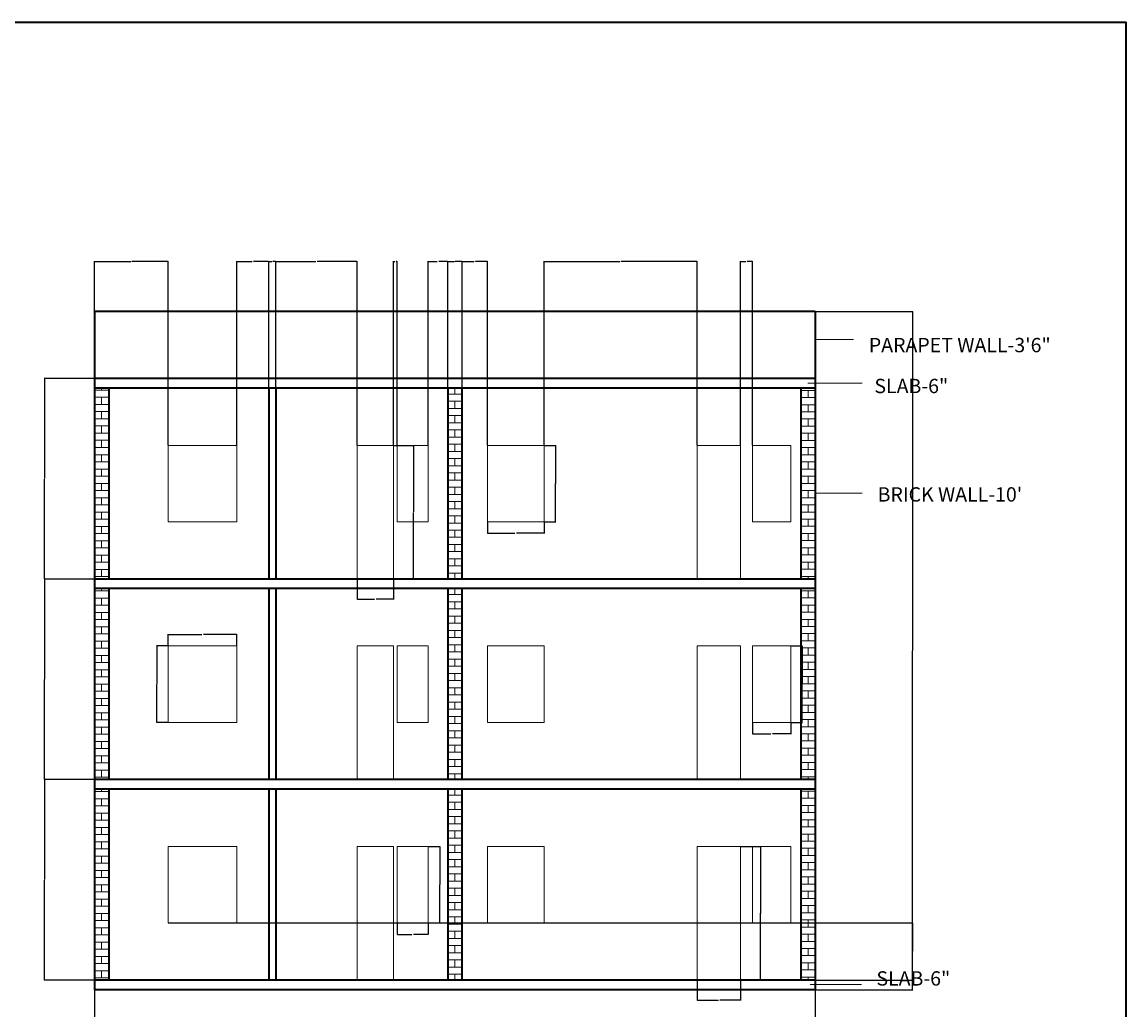
# Model space of a CAD drawing. Units: inches. Extents: x 2250 to 3629, y 982 to 2740.
# Tile 12 of 12: x 2936 to 3629, y 2119 to 2740. Entities that reach past the tile are written whole.
import ezdxf

# ---------------------------------------------------------------- set-up
doc = ezdxf.new("R2010")
doc.units = ezdxf.units.IN
for name, color, linetype, lineweight in [('A-ANNO-DIMS', 2, 'Continuous', 18), ('A-ANNO-TEXT', 7, 'Continuous', 18), ('A-ANNO-TTLB', 7, 'Continuous', 35), ('A-SECT', 7, 'Continuous', 35), ('A-SECT-DOOR', 3, 'Continuous', 18), ('A-SECT-GLAZ', 4, 'Continuous', 18), ('A-WALL-PATT', 252, 'Continuous', 13)]:
    doc.layers.add(name, color=color, linetype=linetype, lineweight=lineweight)
doc.styles.get("Standard").update_dxf_attribs({"font": 'arial.ttf'})
doc.dimstyles.get("Standard").update_dxf_attribs({"dimtxt": 0.18, "dimasz": 0.18, "dimexe": 0.18, "dimexo": 0.0625, "dimgap": 0.09, "dimtad": 0, "dimtih": 1, "dimtoh": 1, "dimdec": 4, "dimzin": 0, "dimdsep": 46, "dimtxsty": 'Standard', "dimcen": 0.09, "dimadec": 0, "dimazin": 0, "dimtfac": 1, "dimtdec": 4, "dimtofl": 0, "dimtmove": 0, "dimatfit": 3, "dimfxl": 1, "dimtolj": 1, "dimtzin": 0, "dimarcsym": 0})

# ---------------------------------------------------------------- blocks, each defined once
blk = doc.blocks.new('SEC-WIN-24x48')
for p, q in [((0, 48), (0, 0)), ((24, 48), (0, 48)), ((24, 48), (24, 0)), ((24, 0), (0, 0))]:
    blk.add_line(p, q)
blk = doc.blocks.new('SEC-WIN-35p52x48')
for p, q in [((0, 48), (0, 0)), ((35.52, 48), (0, 48)), ((35.52, 48), (35.52, 0)), ((35.52, 0), (0, 0))]:
    blk.add_line(p, q)
blk = doc.blocks.new('SEC-WIN-19p52x48')
for p, q in [((0, 48), (0, 0)), ((19.52, 48), (0, 48)), ((19.52, 48), (19.52, 0)), ((19.52, 0), (0, 0))]:
    blk.add_line(p, q)
blk = doc.blocks.new('SEC-WIN-43p24x48')
for p, q in [((0, 48), (0, 0)), ((43.24, 48), (0, 48)), ((43.24, 48), (43.24, 0)), ((43.24, 0), (0, 0))]:
    blk.add_line(p, q)
blk = doc.blocks.new('SEC-DOOR-27p25x84')
for p, q in [((0, 84), (0, 0)), ((27.25, 84), (0, 84)), ((27.25, 84), (27.25, 0))]:
    blk.add_line(p, q)
blk = doc.blocks.new('SEC-DOOR-22p88x84')
for p, q in [((0, 84), (0, 0)), ((22.88, 84), (0, 84)), ((22.88, 84), (22.88, 0))]:
    blk.add_line(p, q)
blk = doc.blocks.new('*D157')
at = {"layer": 'A-ANNO-DIMS', "color": 0, "lineweight": -2, "transparency": 16777216}
for p, q in [((3418.84, 2347.7), (3426.15, 2347.7)), ((3425.97, 2347.52), (3425.97, 2323.88)), ((3425.97, 2299.88), (3425.97, 2323.52)), ((3418.84, 2299.7), (3426.15, 2299.7))]:
    blk.add_line(p, q, dxfattribs=at)
at = {"layer": 'A-ANNO-DIMS', "color": 0, "transparency": 16777216}
for points in [[(3425.94, 2347.52), (3426, 2347.52), (3425.97, 2347.7)], [(3425.94, 2299.88), (3426, 2299.88), (3425.97, 2299.7)]]:
    blk.add_solid(points, dxfattribs=at)
at = {"layer": 'Defpoints', "color": 0, "transparency": 16777216}
for p in [(3418.77, 2347.7), (3425.97, 2347.7), (3418.77, 2299.7)]:
    blk.add_point(p, dxfattribs=at)
at = {"layer": 'A-ANNO-DIMS', "color": 0, "transparency": 16777216, "insert": (3425.97, 2323.7), "char_height": 0.18, "attachment_point": 5}
blk.add_mtext('\\A1;WINDOW 48 TYP.', dxfattribs=at)
blk = doc.blocks.new('*D158')
at = {"layer": 'A-ANNO-DIMS', "color": 0, "lineweight": -2, "transparency": 16777216}
for p, q in [((3394.77, 2299.64), (3394.77, 2292.32)), ((3418.77, 2299.64), (3418.77, 2292.32)), ((3394.95, 2292.5), (3406.24, 2292.5)), ((3418.59, 2292.5), (3407.3, 2292.5))]:
    blk.add_line(p, q, dxfattribs=at)
at = {"layer": 'A-ANNO-DIMS', "color": 0, "transparency": 16777216}
for points in [[(3394.95, 2292.53), (3394.95, 2292.47), (3394.77, 2292.5)], [(3418.59, 2292.53), (3418.59, 2292.47), (3418.77, 2292.5)]]:
    blk.add_solid(points, dxfattribs=at)
at = {"layer": 'Defpoints', "color": 0, "transparency": 16777216}
for p in [(3394.77, 2299.7), (3418.77, 2299.7), (3418.77, 2292.5)]:
    blk.add_point(p, dxfattribs=at)
at = {"layer": 'A-ANNO-DIMS', "color": 0, "transparency": 16777216, "insert": (3406.77, 2292.5), "char_height": 0.18, "attachment_point": 5}
blk.add_mtext('\\A1;24 TYP.', dxfattribs=at)
blk = doc.blocks.new('*D159')
at = {"layer": 'A-ANNO-DIMS', "color": 0, "lineweight": -2, "transparency": 16777216}
for p, q in [((3263.8, 2473.7), (3271.12, 2473.7)), ((3270.94, 2473.52), (3270.94, 2449.88)), ((3270.94, 2425.88), (3270.94, 2449.52)), ((3263.8, 2425.7), (3271.12, 2425.7))]:
    blk.add_line(p, q, dxfattribs=at)
at = {"layer": 'A-ANNO-DIMS', "color": 0, "transparency": 16777216}
for points in [[(3270.91, 2473.52), (3270.97, 2473.52), (3270.94, 2473.7)], [(3270.91, 2425.88), (3270.97, 2425.88), (3270.94, 2425.7)]]:
    blk.add_solid(points, dxfattribs=at)
at = {"layer": 'Defpoints', "color": 0, "transparency": 16777216}
for p in [(3263.74, 2473.7), (3270.94, 2473.7), (3263.74, 2425.7)]:
    blk.add_point(p, dxfattribs=at)
at = {"layer": 'A-ANNO-DIMS', "color": 0, "transparency": 16777216, "insert": (3270.94, 2449.7), "char_height": 0.18, "attachment_point": 5}
blk.add_mtext('\\A1;WINDOW 48 TYP.', dxfattribs=at)
blk = doc.blocks.new('*D160')
at = {"layer": 'A-ANNO-DIMS', "color": 0, "lineweight": -2, "transparency": 16777216}
for p, q in [((3228.22, 2425.64), (3228.22, 2418.32)), ((3263.74, 2425.64), (3263.74, 2418.32)), ((3228.4, 2418.5), (3245.45, 2418.5)), ((3263.56, 2418.5), (3246.51, 2418.5))]:
    blk.add_line(p, q, dxfattribs=at)
at = {"layer": 'A-ANNO-DIMS', "color": 0, "transparency": 16777216}
for points in [[(3228.4, 2418.53), (3228.4, 2418.47), (3228.22, 2418.5)], [(3263.56, 2418.53), (3263.56, 2418.47), (3263.74, 2418.5)]]:
    blk.add_solid(points, dxfattribs=at)
at = {"layer": 'Defpoints', "color": 0, "transparency": 16777216}
for p in [(3228.22, 2425.7), (3263.74, 2425.7), (3263.74, 2418.5)]:
    blk.add_point(p, dxfattribs=at)
at = {"layer": 'A-ANNO-DIMS', "color": 0, "transparency": 16777216, "insert": (3245.98, 2418.5), "char_height": 0.18, "attachment_point": 5}
blk.add_mtext('\\A1;36 TYP.', dxfattribs=at)
blk = doc.blocks.new('*D161')
at = {"layer": 'A-ANNO-DIMS', "color": 0, "lineweight": -2, "transparency": 16777216}
for p, q in [((3191.07, 2221.7), (3198.39, 2221.7)), ((3198.21, 2221.52), (3198.21, 2197.88)), ((3198.21, 2173.88), (3198.21, 2197.52)), ((3191.07, 2173.7), (3198.39, 2173.7))]:
    blk.add_line(p, q, dxfattribs=at)
at = {"layer": 'A-ANNO-DIMS', "color": 0, "transparency": 16777216}
for points in [[(3198.18, 2221.52), (3198.24, 2221.52), (3198.21, 2221.7)], [(3198.18, 2173.88), (3198.24, 2173.88), (3198.21, 2173.7)]]:
    blk.add_solid(points, dxfattribs=at)
at = {"layer": 'Defpoints', "color": 0, "transparency": 16777216}
for p in [(3191.01, 2221.7), (3198.21, 2221.7), (3191.01, 2173.7)]:
    blk.add_point(p, dxfattribs=at)
at = {"layer": 'A-ANNO-DIMS', "color": 0, "transparency": 16777216, "insert": (3198.21, 2197.7), "char_height": 0.18, "attachment_point": 5}
blk.add_mtext('\\A1;WINDOW 48 TYP.', dxfattribs=at)
blk = doc.blocks.new('*D162')
at = {"layer": 'A-ANNO-DIMS', "color": 0, "lineweight": -2, "transparency": 16777216}
for p, q in [((3171.49, 2173.64), (3171.49, 2166.32)), ((3191.01, 2173.64), (3191.01, 2166.32)), ((3171.67, 2166.5), (3180.72, 2166.5)), ((3190.83, 2166.5), (3181.78, 2166.5))]:
    blk.add_line(p, q, dxfattribs=at)
at = {"layer": 'A-ANNO-DIMS', "color": 0, "transparency": 16777216}
for points in [[(3171.67, 2166.53), (3171.67, 2166.47), (3171.49, 2166.5)], [(3190.83, 2166.53), (3190.83, 2166.47), (3191.01, 2166.5)]]:
    blk.add_solid(points, dxfattribs=at)
at = {"layer": 'Defpoints', "color": 0, "transparency": 16777216}
for p in [(3171.49, 2173.7), (3191.01, 2173.7), (3191.01, 2166.5)]:
    blk.add_point(p, dxfattribs=at)
at = {"layer": 'A-ANNO-DIMS', "color": 0, "transparency": 16777216, "insert": (3181.25, 2166.5), "char_height": 0.18, "attachment_point": 5}
blk.add_mtext('\\A1;20 TYP.', dxfattribs=at)
blk = doc.blocks.new('*D163')
at = {"layer": 'A-ANNO-DIMS', "color": 0, "lineweight": -2, "transparency": 16777216}
for p, q in [((3027.45, 2347.7), (3020.13, 2347.7)), ((3020.31, 2347.52), (3020.31, 2323.88)), ((3020.31, 2299.88), (3020.31, 2323.52)), ((3027.45, 2299.7), (3020.13, 2299.7))]:
    blk.add_line(p, q, dxfattribs=at)
at = {"layer": 'A-ANNO-DIMS', "color": 0, "transparency": 16777216}
for points in [[(3020.28, 2347.52), (3020.34, 2347.52), (3020.31, 2347.7)], [(3020.28, 2299.88), (3020.34, 2299.88), (3020.31, 2299.7)]]:
    blk.add_solid(points, dxfattribs=at)
at = {"layer": 'Defpoints', "color": 0, "transparency": 16777216}
for p in [(3027.51, 2347.7), (3020.31, 2299.7), (3027.51, 2299.7)]:
    blk.add_point(p, dxfattribs=at)
at = {"layer": 'A-ANNO-DIMS', "color": 0, "transparency": 16777216, "insert": (3020.31, 2323.7), "char_height": 0.18, "attachment_point": 5}
blk.add_mtext('\\A1;WINDOW 48 TYP.', dxfattribs=at)
blk = doc.blocks.new('*D164')
at = {"layer": 'A-ANNO-DIMS', "color": 0, "lineweight": -2, "transparency": 16777216}
for p, q in [((3027.51, 2347.76), (3027.51, 2355.08)), ((3027.69, 2354.9), (3048.6, 2354.9)), ((3070.58, 2354.9), (3049.67, 2354.9)), ((3070.76, 2347.76), (3070.76, 2355.08))]:
    blk.add_line(p, q, dxfattribs=at)
at = {"layer": 'A-ANNO-DIMS', "color": 0, "transparency": 16777216}
for points in [[(3027.69, 2354.93), (3027.69, 2354.87), (3027.51, 2354.9)], [(3070.58, 2354.93), (3070.58, 2354.87), (3070.76, 2354.9)]]:
    blk.add_solid(points, dxfattribs=at)
at = {"layer": 'Defpoints', "color": 0, "transparency": 16777216}
for p in [(3027.51, 2354.9), (3027.51, 2347.7), (3070.76, 2347.7)]:
    blk.add_point(p, dxfattribs=at)
at = {"layer": 'A-ANNO-DIMS', "color": 0, "transparency": 16777216, "insert": (3049.14, 2354.9), "char_height": 0.18, "attachment_point": 5}
blk.add_mtext('\\A1;43 TYP.', dxfattribs=at)
blk = doc.blocks.new('*D165')
at = {"layer": 'A-ANNO-DIMS', "color": 0, "lineweight": -2, "transparency": 16777216}
for p, q in [((3387.34, 2221.7), (3400.06, 2221.7)), ((3399.88, 2221.52), (3399.88, 2179.88)), ((3399.88, 2137.88), (3399.88, 2179.52)), ((3387.34, 2137.7), (3400.06, 2137.7))]:
    blk.add_line(p, q, dxfattribs=at)
at = {"layer": 'A-ANNO-DIMS', "color": 0, "transparency": 16777216}
for points in [[(3399.85, 2221.52), (3399.91, 2221.52), (3399.88, 2221.7)], [(3399.85, 2137.88), (3399.91, 2137.88), (3399.88, 2137.7)]]:
    blk.add_solid(points, dxfattribs=at)
at = {"layer": 'Defpoints', "color": 0, "transparency": 16777216}
for p in [(3387.28, 2221.7), (3399.88, 2221.7), (3387.28, 2137.7)]:
    blk.add_point(p, dxfattribs=at)
at = {"layer": 'A-ANNO-DIMS', "color": 0, "transparency": 16777216, "insert": (3399.88, 2179.7), "char_height": 0.18, "attachment_point": 5}
blk.add_mtext('\\A1;DOOR 84 TYP.', dxfattribs=at)
blk = doc.blocks.new('*D166')
at = {"layer": 'A-ANNO-DIMS', "color": 0, "lineweight": -2, "transparency": 16777216}
for p, q in [((3360.02, 2137.64), (3360.02, 2124.92)), ((3387.28, 2137.64), (3387.28, 2124.92)), ((3360.2, 2125.1), (3373.12, 2125.1)), ((3387.1, 2125.1), (3374.18, 2125.1))]:
    blk.add_line(p, q, dxfattribs=at)
at = {"layer": 'A-ANNO-DIMS', "color": 0, "transparency": 16777216}
for points in [[(3360.2, 2125.13), (3360.2, 2125.07), (3360.02, 2125.1)], [(3387.1, 2125.13), (3387.1, 2125.07), (3387.28, 2125.1)]]:
    blk.add_solid(points, dxfattribs=at)
at = {"layer": 'Defpoints', "color": 0, "transparency": 16777216}
for p in [(3360.02, 2137.7), (3387.28, 2137.7), (3387.28, 2125.1)]:
    blk.add_point(p, dxfattribs=at)
at = {"layer": 'A-ANNO-DIMS', "color": 0, "transparency": 16777216, "insert": (3373.65, 2125.1), "char_height": 0.18, "attachment_point": 5}
blk.add_mtext('\\A1;27 TYP.', dxfattribs=at)
blk = doc.blocks.new('*D167')
at = {"layer": 'A-ANNO-DIMS', "color": 0, "lineweight": -2, "transparency": 16777216}
for p, q in [((3169.27, 2473.7), (3181.99, 2473.7)), ((3181.81, 2473.52), (3181.81, 2431.88)), ((3181.81, 2389.88), (3181.81, 2431.52)), ((3169.27, 2389.7), (3181.99, 2389.7))]:
    blk.add_line(p, q, dxfattribs=at)
at = {"layer": 'A-ANNO-DIMS', "color": 0, "transparency": 16777216}
for points in [[(3181.78, 2473.52), (3181.84, 2473.52), (3181.81, 2473.7)], [(3181.78, 2389.88), (3181.84, 2389.88), (3181.81, 2389.7)]]:
    blk.add_solid(points, dxfattribs=at)
at = {"layer": 'Defpoints', "color": 0, "transparency": 16777216}
for p in [(3169.21, 2473.7), (3181.81, 2473.7), (3169.21, 2389.7)]:
    blk.add_point(p, dxfattribs=at)
at = {"layer": 'A-ANNO-DIMS', "color": 0, "transparency": 16777216, "insert": (3181.81, 2431.7), "char_height": 0.18, "attachment_point": 5}
blk.add_mtext('\\A1;DOOR 84 TYP.', dxfattribs=at)
blk = doc.blocks.new('*D168')
at = {"layer": 'A-ANNO-DIMS', "color": 0, "lineweight": -2, "transparency": 16777216}
for p, q in [((3146.34, 2389.64), (3146.34, 2376.92)), ((3169.21, 2389.64), (3169.21, 2376.92)), ((3146.52, 2377.1), (3157.24, 2377.1)), ((3169.03, 2377.1), (3158.3, 2377.1))]:
    blk.add_line(p, q, dxfattribs=at)
at = {"layer": 'A-ANNO-DIMS', "color": 0, "transparency": 16777216}
for points in [[(3146.52, 2377.13), (3146.52, 2377.07), (3146.34, 2377.1)], [(3169.03, 2377.13), (3169.03, 2377.07), (3169.21, 2377.1)]]:
    blk.add_solid(points, dxfattribs=at)
at = {"layer": 'Defpoints', "color": 0, "transparency": 16777216}
for p in [(3146.34, 2389.7), (3169.21, 2389.7), (3169.21, 2377.1)]:
    blk.add_point(p, dxfattribs=at)
at = {"layer": 'A-ANNO-DIMS', "color": 0, "transparency": 16777216, "insert": (3157.77, 2377.1), "char_height": 0.18, "attachment_point": 5}
blk.add_mtext('\\A1;23 TYP.', dxfattribs=at)
blk = doc.blocks.new('*D188')
at = {"layer": 'A-ANNO-DIMS', "color": 0, "lineweight": -2, "transparency": 16777216}
for p, q in [((2981.23, 2131.64), (2981.23, 2056.9)), ((3434.23, 2131.64), (3434.23, 2056.9)), ((2981.41, 2057.08), (3207.43, 2057.08)), ((3434.05, 2057.08), (3208.02, 2057.08))]:
    blk.add_line(p, q, dxfattribs=at)
at = {"layer": 'A-ANNO-DIMS', "color": 0, "transparency": 16777216}
for points in [[(2981.41, 2057.11), (2981.41, 2057.05), (2981.23, 2057.08)], [(3434.05, 2057.11), (3434.05, 2057.05), (3434.23, 2057.08)]]:
    blk.add_solid(points, dxfattribs=at)
at = {"layer": 'Defpoints', "color": 0, "transparency": 16777216}
for p in [(2981.23, 2131.7), (3434.23, 2131.7), (3434.23, 2057.08)]:
    blk.add_point(p, dxfattribs=at)
at = {"layer": 'A-ANNO-DIMS', "color": 0, "transparency": 16777216, "insert": (3207.73, 2057.08), "char_height": 0.18, "attachment_point": 5}
blk.add_mtext('\\A1;453', dxfattribs=at)
blk = doc.blocks.new('*D189')
at = {"layer": 'A-ANNO-DIMS', "color": 0, "lineweight": -2, "transparency": 16777216}
for p, q in [((3434.29, 2557.7), (3495.46, 2557.7)), ((3495.28, 2557.52), (3495.28, 2344.88)), ((3495.28, 2131.88), (3495.28, 2344.52)), ((3434.29, 2131.7), (3495.46, 2131.7))]:
    blk.add_line(p, q, dxfattribs=at)
at = {"layer": 'A-ANNO-DIMS', "color": 0, "transparency": 16777216}
for points in [[(3495.25, 2557.52), (3495.31, 2557.52), (3495.28, 2557.7)], [(3495.25, 2131.88), (3495.31, 2131.88), (3495.28, 2131.7)]]:
    blk.add_solid(points, dxfattribs=at)
at = {"layer": 'Defpoints', "color": 0, "transparency": 16777216}
for p in [(3434.23, 2557.7), (3495.28, 2557.7), (3434.23, 2131.7)]:
    blk.add_point(p, dxfattribs=at)
at = {"layer": 'A-ANNO-DIMS', "color": 0, "transparency": 16777216, "insert": (3495.28, 2344.7), "char_height": 0.18, "attachment_point": 5}
blk.add_mtext('\\A1;426', dxfattribs=at)
blk = doc.blocks.new('*D190')
at = {"layer": 'A-ANNO-DIMS', "color": 0, "lineweight": -2, "transparency": 16777216}
for p, q in [((2981.16, 2263.7), (2949.55, 2263.7)), ((2949.73, 2263.52), (2949.73, 2200.88)), ((2949.73, 2137.88), (2949.73, 2200.52)), ((2981.16, 2137.7), (2949.55, 2137.7))]:
    blk.add_line(p, q, dxfattribs=at)
at = {"layer": 'A-ANNO-DIMS', "color": 0, "transparency": 16777216}
for points in [[(2949.7, 2263.52), (2949.76, 2263.52), (2949.73, 2263.7)], [(2949.7, 2137.88), (2949.76, 2137.88), (2949.73, 2137.7)]]:
    blk.add_solid(points, dxfattribs=at)
at = {"layer": 'Defpoints', "color": 0, "transparency": 16777216}
for p in [(2949.73, 2263.7), (2981.23, 2263.7), (2981.23, 2137.7)]:
    blk.add_point(p, dxfattribs=at)
at = {"layer": 'A-ANNO-DIMS', "color": 0, "transparency": 16777216, "insert": (2949.73, 2200.7), "char_height": 0.18, "attachment_point": 5}
blk.add_mtext('\\A1;126', dxfattribs=at)
blk = doc.blocks.new('*D191')
at = {"layer": 'A-ANNO-DIMS', "color": 0, "lineweight": -2, "transparency": 16777216}
for p, q in [((2981.16, 2389.7), (2949.55, 2389.7)), ((2949.73, 2389.52), (2949.73, 2326.88)), ((2949.73, 2263.88), (2949.73, 2326.52)), ((2981.16, 2263.7), (2949.55, 2263.7))]:
    blk.add_line(p, q, dxfattribs=at)
at = {"layer": 'A-ANNO-DIMS', "color": 0, "transparency": 16777216}
for points in [[(2949.7, 2389.52), (2949.76, 2389.52), (2949.73, 2389.7)], [(2949.7, 2263.88), (2949.76, 2263.88), (2949.73, 2263.7)]]:
    blk.add_solid(points, dxfattribs=at)
at = {"layer": 'Defpoints', "color": 0, "transparency": 16777216}
for p in [(2949.73, 2389.7), (2981.23, 2389.7), (2981.23, 2263.7)]:
    blk.add_point(p, dxfattribs=at)
at = {"layer": 'A-ANNO-DIMS', "color": 0, "transparency": 16777216, "insert": (2949.73, 2326.7), "char_height": 0.18, "attachment_point": 5}
blk.add_mtext('\\A1;126', dxfattribs=at)
blk = doc.blocks.new('*D192')
at = {"layer": 'A-ANNO-DIMS', "color": 0, "lineweight": -2, "transparency": 16777216}
for p, q in [((2981.16, 2515.7), (2949.55, 2515.7)), ((2949.73, 2515.52), (2949.73, 2452.88)), ((2949.73, 2389.88), (2949.73, 2452.52)), ((2981.16, 2389.7), (2949.55, 2389.7))]:
    blk.add_line(p, q, dxfattribs=at)
at = {"layer": 'A-ANNO-DIMS', "color": 0, "transparency": 16777216}
for points in [[(2949.7, 2515.52), (2949.76, 2515.52), (2949.73, 2515.7)], [(2949.7, 2389.88), (2949.76, 2389.88), (2949.73, 2389.7)]]:
    blk.add_solid(points, dxfattribs=at)
at = {"layer": 'Defpoints', "color": 0, "transparency": 16777216}
for p in [(2949.73, 2515.7), (2981.23, 2515.7), (2981.23, 2389.7)]:
    blk.add_point(p, dxfattribs=at)
at = {"layer": 'A-ANNO-DIMS', "color": 0, "transparency": 16777216, "insert": (2949.73, 2452.7), "char_height": 0.18, "attachment_point": 5}
blk.add_mtext('\\A1;126', dxfattribs=at)
blk = doc.blocks.new('*D193')
at = {"layer": 'A-ANNO-DIMS', "color": 0, "lineweight": -2, "transparency": 16777216}
for p, q in [((3027.58, 2173.7), (3495.46, 2173.7)), ((3495.28, 2173.52), (3495.28, 2155.88)), ((3495.28, 2137.88), (3495.28, 2155.52)), ((2990.29, 2137.7), (3495.46, 2137.7))]:
    blk.add_line(p, q, dxfattribs=at)
at = {"layer": 'A-ANNO-DIMS', "color": 0, "transparency": 16777216}
for points in [[(3495.25, 2173.52), (3495.31, 2173.52), (3495.28, 2173.7)], [(3495.25, 2137.88), (3495.31, 2137.88), (3495.28, 2137.7)]]:
    blk.add_solid(points, dxfattribs=at)
at = {"layer": 'Defpoints', "color": 0, "transparency": 16777216}
for p in [(3027.51, 2173.7), (2990.23, 2137.7), (3495.28, 2137.7)]:
    blk.add_point(p, dxfattribs=at)
at = {"layer": 'A-ANNO-DIMS', "color": 0, "transparency": 16777216, "insert": (3495.28, 2155.7), "char_height": 0.18, "attachment_point": 5}
blk.add_mtext('\\A1;36', dxfattribs=at)
blk = doc.blocks.new('*D194')
at = {"layer": 'A-ANNO-DIMS', "color": 0, "lineweight": -2, "transparency": 16777216}
for p, q in [((2981.23, 2509.76), (2981.23, 2589.38)), ((2981.41, 2589.2), (3003.97, 2589.2)), ((3027.33, 2589.2), (3004.77, 2589.2)), ((3027.51, 2473.76), (3027.51, 2589.38))]:
    blk.add_line(p, q, dxfattribs=at)
at = {"layer": 'A-ANNO-DIMS', "color": 0, "transparency": 16777216}
for points in [[(2981.41, 2589.23), (2981.41, 2589.17), (2981.23, 2589.2)], [(3027.33, 2589.23), (3027.33, 2589.17), (3027.51, 2589.2)]]:
    blk.add_solid(points, dxfattribs=at)
at = {"layer": 'Defpoints', "color": 0, "transparency": 16777216}
for p in [(3027.51, 2589.2), (2981.23, 2509.7), (3027.51, 2473.7)]:
    blk.add_point(p, dxfattribs=at)
at = {"layer": 'A-ANNO-DIMS', "color": 0, "transparency": 16777216, "insert": (3004.37, 2589.2), "char_height": 0.18, "attachment_point": 5}
blk.add_mtext('\\A1;46.29', dxfattribs=at)
blk = doc.blocks.new('*D195')
at = {"layer": 'A-ANNO-DIMS', "color": 0, "lineweight": -2, "transparency": 16777216}
for p, q in [((3070.76, 2473.76), (3070.76, 2589.38)), ((3070.94, 2589.2), (3080.36, 2589.2)), ((3090.55, 2589.2), (3081.13, 2589.2)), ((3090.73, 2509.76), (3090.73, 2589.38))]:
    blk.add_line(p, q, dxfattribs=at)
at = {"layer": 'A-ANNO-DIMS', "color": 0, "transparency": 16777216}
for points in [[(3070.94, 2589.23), (3070.94, 2589.17), (3070.76, 2589.2)], [(3090.55, 2589.23), (3090.55, 2589.17), (3090.73, 2589.2)]]:
    blk.add_solid(points, dxfattribs=at)
at = {"layer": 'Defpoints', "color": 0, "transparency": 16777216}
for p in [(3090.73, 2589.2), (3090.73, 2509.7), (3070.76, 2473.7)]:
    blk.add_point(p, dxfattribs=at)
at = {"layer": 'A-ANNO-DIMS', "color": 0, "transparency": 16777216, "insert": (3080.74, 2589.2), "char_height": 0.18, "attachment_point": 5}
blk.add_mtext('\\A1;19.97', dxfattribs=at)
blk = doc.blocks.new('*D196')
at = {"layer": 'A-ANNO-DIMS', "color": 0, "lineweight": -2, "transparency": 16777216}
for p, q in [((3090.73, 2509.76), (3090.73, 2589.38)), ((3090.91, 2589.2), (3092.72, 2589.2)), ((3095.05, 2589.2), (3093.23, 2589.2)), ((3095.23, 2509.76), (3095.23, 2589.38))]:
    blk.add_line(p, q, dxfattribs=at)
at = {"layer": 'A-ANNO-DIMS', "color": 0, "transparency": 16777216}
for points in [[(3090.91, 2589.23), (3090.91, 2589.17), (3090.73, 2589.2)], [(3095.05, 2589.23), (3095.05, 2589.17), (3095.23, 2589.2)]]:
    blk.add_solid(points, dxfattribs=at)
at = {"layer": 'Defpoints', "color": 0, "transparency": 16777216}
for p in [(3095.23, 2589.2), (3090.73, 2509.7), (3095.23, 2509.7)]:
    blk.add_point(p, dxfattribs=at)
at = {"layer": 'A-ANNO-DIMS', "color": 0, "transparency": 16777216, "insert": (3092.98, 2589.2), "char_height": 0.18, "attachment_point": 5}
blk.add_mtext('\\A1;4.5', dxfattribs=at)
blk = doc.blocks.new('*D197')
at = {"layer": 'A-ANNO-DIMS', "color": 0, "lineweight": -2, "transparency": 16777216}
for p, q in [((3095.23, 2509.76), (3095.23, 2589.38)), ((3095.41, 2589.2), (3120.41, 2589.2)), ((3146.16, 2589.2), (3121.16, 2589.2)), ((3146.34, 2473.76), (3146.34, 2589.38))]:
    blk.add_line(p, q, dxfattribs=at)
at = {"layer": 'A-ANNO-DIMS', "color": 0, "transparency": 16777216}
for points in [[(3095.41, 2589.23), (3095.41, 2589.17), (3095.23, 2589.2)], [(3146.16, 2589.23), (3146.16, 2589.17), (3146.34, 2589.2)]]:
    blk.add_solid(points, dxfattribs=at)
at = {"layer": 'Defpoints', "color": 0, "transparency": 16777216}
for p in [(3146.34, 2589.2), (3095.23, 2509.7), (3146.34, 2473.7)]:
    blk.add_point(p, dxfattribs=at)
at = {"layer": 'A-ANNO-DIMS', "color": 0, "transparency": 16777216, "insert": (3120.78, 2589.2), "char_height": 0.18, "attachment_point": 5}
blk.add_mtext('\\A1;51.11', dxfattribs=at)
blk = doc.blocks.new('*D198')
at = {"layer": 'A-ANNO-DIMS', "color": 0, "lineweight": -2, "transparency": 16777216}
for p, q in [((3169.21, 2473.76), (3169.21, 2589.38)), ((3169.39, 2589.2), (3169.96, 2589.2)), ((3171.31, 2589.2), (3170.75, 2589.2)), ((3171.49, 2473.76), (3171.49, 2589.38))]:
    blk.add_line(p, q, dxfattribs=at)
at = {"layer": 'A-ANNO-DIMS', "color": 0, "transparency": 16777216}
for points in [[(3169.39, 2589.23), (3169.39, 2589.17), (3169.21, 2589.2)], [(3171.31, 2589.23), (3171.31, 2589.17), (3171.49, 2589.2)]]:
    blk.add_solid(points, dxfattribs=at)
at = {"layer": 'Defpoints', "color": 0, "transparency": 16777216}
for p in [(3171.49, 2589.2), (3169.21, 2473.7), (3171.49, 2473.7)]:
    blk.add_point(p, dxfattribs=at)
at = {"layer": 'A-ANNO-DIMS', "color": 0, "transparency": 16777216, "insert": (3170.35, 2589.2), "char_height": 0.18, "attachment_point": 5}
blk.add_mtext('\\A1;2.278', dxfattribs=at)
blk = doc.blocks.new('*D199')
at = {"layer": 'A-ANNO-DIMS', "color": 0, "lineweight": -2, "transparency": 16777216}
for p, q in [((3191.01, 2473.76), (3191.01, 2589.38)), ((3191.19, 2589.2), (3196.66, 2589.2)), ((3203.05, 2589.2), (3197.57, 2589.2)), ((3203.23, 2509.76), (3203.23, 2589.38))]:
    blk.add_line(p, q, dxfattribs=at)
at = {"layer": 'A-ANNO-DIMS', "color": 0, "transparency": 16777216}
for points in [[(3191.19, 2589.23), (3191.19, 2589.17), (3191.01, 2589.2)], [(3203.05, 2589.23), (3203.05, 2589.17), (3203.23, 2589.2)]]:
    blk.add_solid(points, dxfattribs=at)
at = {"layer": 'Defpoints', "color": 0, "transparency": 16777216}
for p in [(3203.23, 2589.2), (3203.23, 2509.7), (3191.01, 2473.7)]:
    blk.add_point(p, dxfattribs=at)
at = {"layer": 'A-ANNO-DIMS', "color": 0, "transparency": 16777216, "insert": (3197.12, 2589.2), "char_height": 0.18, "attachment_point": 5}
blk.add_mtext('\\A1;12.216', dxfattribs=at)
blk = doc.blocks.new('*D200')
at = {"layer": 'A-ANNO-DIMS', "color": 0, "lineweight": -2, "transparency": 16777216}
for p, q in [((3203.23, 2509.76), (3203.23, 2589.38)), ((3203.41, 2589.2), (3207.58, 2589.2)), ((3212.05, 2589.2), (3207.88, 2589.2)), ((3212.23, 2509.76), (3212.23, 2589.38))]:
    blk.add_line(p, q, dxfattribs=at)
at = {"layer": 'A-ANNO-DIMS', "color": 0, "transparency": 16777216}
for points in [[(3203.41, 2589.23), (3203.41, 2589.17), (3203.23, 2589.2)], [(3212.05, 2589.23), (3212.05, 2589.17), (3212.23, 2589.2)]]:
    blk.add_solid(points, dxfattribs=at)
at = {"layer": 'Defpoints', "color": 0, "transparency": 16777216}
for p in [(3212.23, 2589.2), (3203.23, 2509.7), (3212.23, 2509.7)]:
    blk.add_point(p, dxfattribs=at)
at = {"layer": 'A-ANNO-DIMS', "color": 0, "transparency": 16777216, "insert": (3207.73, 2589.2), "char_height": 0.18, "attachment_point": 5}
blk.add_mtext('\\A1;9', dxfattribs=at)
blk = doc.blocks.new('*D201')
at = {"layer": 'A-ANNO-DIMS', "color": 0, "lineweight": -2, "transparency": 16777216}
for p, q in [((3212.23, 2509.76), (3212.23, 2589.38)), ((3212.41, 2589.2), (3219.84, 2589.2)), ((3228.04, 2589.2), (3220.61, 2589.2)), ((3228.22, 2473.76), (3228.22, 2589.38))]:
    blk.add_line(p, q, dxfattribs=at)
at = {"layer": 'A-ANNO-DIMS', "color": 0, "transparency": 16777216}
for points in [[(3212.41, 2589.23), (3212.41, 2589.17), (3212.23, 2589.2)], [(3228.04, 2589.23), (3228.04, 2589.17), (3228.22, 2589.2)]]:
    blk.add_solid(points, dxfattribs=at)
at = {"layer": 'Defpoints', "color": 0, "transparency": 16777216}
for p in [(3228.22, 2589.2), (3212.23, 2509.7), (3228.22, 2473.7)]:
    blk.add_point(p, dxfattribs=at)
at = {"layer": 'A-ANNO-DIMS', "color": 0, "transparency": 16777216, "insert": (3220.22, 2589.2), "char_height": 0.18, "attachment_point": 5}
blk.add_mtext('\\A1;15.99', dxfattribs=at)
blk = doc.blocks.new('*D202')
at = {"layer": 'A-ANNO-DIMS', "color": 0, "lineweight": -2, "transparency": 16777216}
for p, q in [((3263.74, 2473.76), (3263.74, 2589.38)), ((3263.92, 2589.2), (3311.49, 2589.2)), ((3359.84, 2589.2), (3312.27, 2589.2)), ((3360.02, 2473.76), (3360.02, 2589.38))]:
    blk.add_line(p, q, dxfattribs=at)
at = {"layer": 'A-ANNO-DIMS', "color": 0, "transparency": 16777216}
for points in [[(3263.92, 2589.23), (3263.92, 2589.17), (3263.74, 2589.2)], [(3359.84, 2589.23), (3359.84, 2589.17), (3360.02, 2589.2)]]:
    blk.add_solid(points, dxfattribs=at)
at = {"layer": 'Defpoints', "color": 0, "transparency": 16777216}
for p in [(3360.02, 2589.2), (3263.74, 2473.7), (3360.02, 2473.7)]:
    blk.add_point(p, dxfattribs=at)
at = {"layer": 'A-ANNO-DIMS', "color": 0, "transparency": 16777216, "insert": (3311.88, 2589.2), "char_height": 0.18, "attachment_point": 5}
blk.add_mtext('\\A1;96.28', dxfattribs=at)
blk = doc.blocks.new('*D203')
at = {"layer": 'A-ANNO-DIMS', "color": 0, "lineweight": -2, "transparency": 16777216}
for p, q in [((3387.28, 2473.76), (3387.28, 2589.38)), ((3387.46, 2589.2), (3390.63, 2589.2)), ((3394.59, 2589.2), (3391.42, 2589.2)), ((3394.77, 2473.76), (3394.77, 2589.38))]:
    blk.add_line(p, q, dxfattribs=at)
at = {"layer": 'A-ANNO-DIMS', "color": 0, "transparency": 16777216}
for points in [[(3387.46, 2589.23), (3387.46, 2589.17), (3387.28, 2589.2)], [(3394.59, 2589.23), (3394.59, 2589.17), (3394.77, 2589.2)]]:
    blk.add_solid(points, dxfattribs=at)
at = {"layer": 'Defpoints', "color": 0, "transparency": 16777216}
for p in [(3394.77, 2589.2), (3387.28, 2473.7), (3394.77, 2473.7)]:
    blk.add_point(p, dxfattribs=at)
at = {"layer": 'A-ANNO-DIMS', "color": 0, "transparency": 16777216, "insert": (3391.02, 2589.2), "char_height": 0.18, "attachment_point": 5}
blk.add_mtext('\\A1;7.497', dxfattribs=at)

msp = doc.modelspace()

# ---------------------------------------------------------------- hatches: boundary and pattern name
at = {"layer": 'A-WALL-PATT'}
h = msp.add_hatch(dxfattribs=at)
h.set_pattern_fill('BRICK', color=256, scale=0.709191, style=0)
h.paths.add_polyline_path([(2981.2267, 2389.6999), (2990.2267, 2389.6999), (2990.2267, 2509.6999), (2981.2267, 2509.6999)])
h = msp.add_hatch(dxfattribs=at)
h.set_pattern_fill('BRICK', color=256, scale=0.70849, style=0)
h.paths.add_polyline_path([(3203.2267, 2389.6999), (3212.2267, 2389.6999), (3212.2267, 2509.6999), (3203.2267, 2509.6999)])
h = msp.add_hatch(dxfattribs=at)
h.set_pattern_fill('BRICK', color=256, scale=0.707882, style=0)
h.paths.add_polyline_path([(3425.2267, 2389.6999), (3434.2267, 2389.6999), (3434.2267, 2509.6999), (3425.2267, 2509.6999)])
h = msp.add_hatch(dxfattribs=at)
h.set_pattern_fill('BRICK', color=256, scale=0.709191, style=0)
h.paths.add_polyline_path([(2981.2267, 2263.6999), (2990.2267, 2263.6999), (2990.2267, 2383.6999), (2981.2267, 2383.6999)])
h = msp.add_hatch(dxfattribs=at)
h.set_pattern_fill('BRICK', color=256, scale=0.70849, style=0)
h.paths.add_polyline_path([(3203.2267, 2263.6999), (3212.2267, 2263.6999), (3212.2267, 2383.6999), (3203.2267, 2383.6999)])
h = msp.add_hatch(dxfattribs=at)
h.set_pattern_fill('BRICK', color=256, scale=0.707882, style=0)
h.paths.add_polyline_path([(3425.2267, 2263.6999), (3434.2267, 2263.6999), (3434.2267, 2383.6999), (3425.2267, 2383.6999)])
h = msp.add_hatch(dxfattribs=at)
h.set_pattern_fill('BRICK', color=256, scale=0.709191, style=0)
h.paths.add_polyline_path([(2981.2267, 2137.6999), (2990.2267, 2137.6999), (2990.2267, 2257.6999), (2981.2267, 2257.6999)])
h = msp.add_hatch(dxfattribs=at)
h.set_pattern_fill('BRICK', color=256, scale=0.70849, style=0)
h.paths.add_polyline_path([(3203.2267, 2137.6999), (3212.2267, 2137.6999), (3212.2267, 2257.6999), (3203.2267, 2257.6999)])
h = msp.add_hatch(dxfattribs=at)
h.set_pattern_fill('BRICK', color=256, scale=0.707882, style=0)
h.paths.add_polyline_path([(3425.2267, 2137.6999), (3434.2267, 2137.6999), (3434.2267, 2257.6999), (3425.2267, 2257.6999)])

# ---------------------------------------------------------------- linework, layer by layer
at = {"layer": 'A-ANNO-TEXT'}
for p, q in [((3434.2267, 2540.2919), (3458.1583, 2540.2919)), ((3429.5563, 2512.6646), (3463.6397, 2512.6646)), ((3434.2267, 2443.6442), (3463.779, 2443.6442)), ((3431.0104, 2134.9844), (3463.3553, 2134.9844))]:
    msp.add_line(p, q, dxfattribs=at)
at = {"layer": 'A-ANNO-TTLB'}
msp.add_lwpolyline([(2249.6849, 2739.593), (3629.4532, 2739.593), (3629.4532, 982.3108), (2249.6849, 982.3108)], close=True, dxfattribs=at)
at = {"layer": 'A-SECT'}
for p, q in [((2981.2267, 2557.6999), (2981.2267, 2383.6999)), ((3434.2267, 2557.6999), (2981.2267, 2557.6999)), ((3434.2267, 2557.6999), (3434.2267, 2383.6999)), ((3434.2267, 2515.6999), (2981.2267, 2515.6999)), ((3434.2267, 2509.6999), (2981.2267, 2509.6999)), ((2990.2267, 2509.6999), (2990.2267, 2389.6999)), ((3090.7267, 2509.6999), (3090.7267, 2389.6999)), ((3095.2267, 2509.6999), (3095.2267, 2389.6999)), ((3212.2267, 2509.6999), (3203.2267, 2509.6999)), ((3203.2267, 2509.6999), (3203.2267, 2389.6999)), ((3212.2267, 2389.6999), (3212.2267, 2509.6999)), ((3425.2267, 2509.6999), (3425.2267, 2389.6999)), ((2981.2267, 2431.6999), (2981.2267, 2257.6999)), ((3434.2267, 2431.6999), (3434.2267, 2257.6999)), ((3434.2267, 2389.6999), (2981.2267, 2389.6999)), ((3434.2267, 2383.6999), (2981.2267, 2383.6999)), ((2990.2267, 2383.6999), (2990.2267, 2263.6999)), ((3090.7267, 2383.6999), (3090.7267, 2263.6999)), ((3095.2267, 2383.6999), (3095.2267, 2263.6999)), ((3212.2267, 2383.6999), (3203.2267, 2383.6999)), ((3203.2267, 2383.6999), (3203.2267, 2263.6999)), ((3212.2267, 2263.6999), (3212.2267, 2383.6999)), ((3425.2267, 2383.6999), (3425.2267, 2263.6999)), ((2981.2267, 2305.6999), (2981.2267, 2131.6999)), ((3434.2267, 2305.6999), (3434.2267, 2131.6999)), ((3434.2267, 2263.6999), (2981.2267, 2263.6999)), ((3434.2267, 2257.6999), (2981.2267, 2257.6999)), ((2990.2267, 2257.6999), (2990.2267, 2137.6999)), ((3090.7267, 2257.6999), (3090.7267, 2137.6999)), ((3095.2267, 2257.6999), (3095.2267, 2137.6999)), ((3212.2267, 2257.6999), (3203.2267, 2257.6999)), ((3203.2267, 2257.6999), (3203.2267, 2137.6999)), ((3212.2267, 2137.6999), (3212.2267, 2257.6999)), ((3425.2267, 2257.6999), (3425.2267, 2137.6999)), ((3434.2267, 2137.6999), (2981.2267, 2137.6999)), ((3434.2267, 2131.6999), (2981.2267, 2131.6999))]:
    msp.add_line(p, q, dxfattribs=at)

# ---------------------------------------------------------------- block references
at = {"layer": 'A-SECT-DOOR'}
for name, p in [('SEC-DOOR-22p88x84', (3146.336, 2389.7)), ('SEC-DOOR-27p25x84', (3360.022, 2389.7)), ('SEC-DOOR-22p88x84', (3146.336, 2263.7)), ('SEC-DOOR-27p25x84', (3360.022, 2263.7)), ('SEC-DOOR-22p88x84', (3146.336, 2137.7)), ('SEC-DOOR-27p25x84', (3360.022, 2137.7))]:
    msp.add_blockref(name, p, dxfattribs=at)
at = {"layer": 'A-SECT-GLAZ', "rotation": 180}
for p in [(3070.7561, 2473.6998), (3070.7561, 2347.6998)]:
    msp.add_blockref('SEC-WIN-43p24x48', p, dxfattribs=at)
at = {"layer": 'A-SECT-GLAZ'}
for name, p in [('SEC-WIN-19p52x48', (3171.49, 2425.7)), ('SEC-WIN-35p52x48', (3228.218, 2425.7)), ('SEC-WIN-24x48', (3394.773, 2425.7)), ('SEC-WIN-19p52x48', (3171.49, 2299.7)), ('SEC-WIN-35p52x48', (3228.218, 2299.7)), ('SEC-WIN-24x48', (3394.773, 2299.7)), ('SEC-WIN-43p24x48', (3027.514, 2173.7)), ('SEC-WIN-19p52x48', (3171.49, 2173.7)), ('SEC-WIN-35p52x48', (3228.218, 2173.7)), ('SEC-WIN-24x48', (3394.773, 2173.7))]:
    msp.add_blockref(name, p, dxfattribs=at)

# ---------------------------------------------------------------- texts
at = {"layer": 'A-ANNO-TEXT', "char_height": 9, "attachment_point": 1}
for s, width, insert in [('PARAPET WALL-3\'6"', 190.524189, (3467.879, 2541.1928)), ('SLAB-6"', 52.4774, (3471.3752, 2515.493)), ("BRICK WALL-10'", 171.759734, (3473.4108, 2447.3794)), ('SLAB-6"', 128.130619, (3472.6509, 2143.3281))]:
    msp.add_mtext_dynamic_manual_height_columns(s, width=width, gutter_width=12.5, heights=[0], dxfattribs=dict(at, insert=insert))

# ---------------------------------------------------------------- dimensions: what is measured, and where the dimension line sits
at = {"layer": 'A-ANNO-DIMS'}
for base, p1, p2, override, picture, middle in [((3027.5144, 2589.1999), (2981.2267, 2509.6999), (3027.5144, 2473.6999), {"dimdec": 2, "dimlfac": 1, "dimrnd": 0, "dimzin": 0, "dimdsep": 46, "dimlunit": 2}, '*D194', (3004.3706, 2589.1999)), ((3090.7267, 2589.1999), (3070.7557, 2473.6999), (3090.7267, 2509.6999), {"dimdec": 2, "dimlfac": 1, "dimrnd": 0, "dimzin": 0, "dimdsep": 46, "dimlunit": 2}, '*D195', (3080.7412, 2589.1999)), ((3095.2267, 2589.1999), (3090.7267, 2509.6999), (3095.2267, 2509.6999), {"dimdec": 1, "dimlfac": 1, "dimrnd": 0, "dimzin": 0, "dimdsep": 46, "dimlunit": 2}, '*D196', (3092.9767, 2589.1999)), ((3146.3361, 2589.1999), (3095.2267, 2509.6999), (3146.3361, 2473.6999), {"dimdec": 2, "dimlfac": 1, "dimrnd": 0, "dimzin": 0, "dimdsep": 46, "dimlunit": 2}, '*D197', (3120.7814, 2589.1999)), ((3171.4904, 2589.1999), (3169.2123, 2473.6999), (3171.4904, 2473.6999), {"dimdec": 3, "dimlfac": 1, "dimrnd": 0, "dimzin": 0, "dimdsep": 46, "dimlunit": 2}, '*D198', (3170.3513, 2589.1999)), ((3203.2267, 2589.1999), (3191.0111, 2473.6999), (3203.2267, 2509.6999), {"dimdec": 3, "dimlfac": 1, "dimrnd": 0, "dimzin": 0, "dimdsep": 46, "dimlunit": 2}, '*D199', (3197.1189, 2589.1999)), ((3212.2267, 2589.1999), (3203.2267, 2509.6999), (3212.2267, 2509.6999), {"dimdec": 0, "dimlfac": 1, "dimrnd": 0, "dimzin": 0, "dimdsep": 46, "dimlunit": 2}, '*D200', (3207.7267, 2589.1999)), ((3228.2181, 2589.1999), (3212.2267, 2509.6999), (3228.2181, 2473.6999), {"dimdec": 2, "dimlfac": 1, "dimrnd": 0, "dimzin": 0, "dimdsep": 46, "dimlunit": 2}, '*D201', (3220.2224, 2589.1999)), ((3360.0215, 2589.1999), (3263.7374, 2473.6999), (3360.0215, 2473.6999), {"dimdec": 2, "dimlfac": 1, "dimrnd": 0, "dimzin": 0, "dimdsep": 46, "dimlunit": 2}, '*D202', (3311.8795, 2589.1999)), ((3394.7725, 2589.1999), (3387.2755, 2473.6999), (3394.7725, 2473.6999), {"dimdec": 3, "dimlfac": 1, "dimrnd": 0, "dimzin": 0, "dimdsep": 46, "dimlunit": 2}, '*D203', (3391.024, 2589.1999)), ((3434.2267, 2057.0817), (2981.2267, 2131.6999), (3434.2267, 2131.6999), {"dimdec": 0, "dimlfac": 1, "dimrnd": 0, "dimzin": 0, "dimdsep": 46, "dimlunit": 2}, '*D188', (3207.7267, 2057.0817))]:
    dim = msp.add_linear_dim(base=base, p1=p1, p2=p2, dimstyle='Standard', override=override, dxfattribs=at)
    dim.commit()
    dim.dimension.update_dxf_attribs({"geometry": picture, "text_midpoint": middle})
for base, p1, p2, picture, middle in [((3495.279, 2557.6999), (3434.2267, 2131.6999), (3434.2267, 2557.6999), '*D189', (3495.279, 2344.6999)), ((2949.7267, 2515.6999), (2981.2267, 2389.6999), (2981.2267, 2515.6999), '*D192', (2949.7267, 2452.6999)), ((2949.7267, 2389.6999), (2981.2267, 2263.6999), (2981.2267, 2389.6999), '*D191', (2949.7267, 2326.6999)), ((2949.7267, 2263.6999), (2981.2267, 2137.6999), (2981.2267, 2263.6999), '*D190', (2949.7267, 2200.6999)), ((3495.279, 2137.6999), (3027.5144, 2173.6999), (2990.2267, 2137.6999), '*D193', (3495.279, 2155.6999))]:
    dim = msp.add_linear_dim(base=base, p1=p1, p2=p2, angle=90, dimstyle='Standard', override={"dimdec": 0, "dimlfac": 1, "dimrnd": 0, "dimzin": 0, "dimdsep": 46, "dimlunit": 2}, dxfattribs=at)
    dim.commit()
    dim.dimension.update_dxf_attribs({"geometry": picture, "text_midpoint": middle})
for base, p1, p2, angle, text, picture, middle in [((3181.8123, 2473.6999), (3169.2123, 2389.6999), (3169.2123, 2473.6999), 90, 'DOOR <> TYP.', '*D167', (3181.8123, 2431.6999)), ((3270.9374, 2473.6999), (3263.7374, 2425.6999), (3263.7374, 2473.6999), 90, 'WINDOW <> TYP.', '*D159', (3270.9374, 2449.6999)), ((3027.5144, 2354.8999), (3070.7557, 2347.6999), (3027.5144, 2347.6999), 180, '<> TYP.', '*D164', (3049.135, 2354.8999)), ((3020.3144, 2299.6999), (3027.5144, 2347.6999), (3027.5144, 2299.6999), 270, 'WINDOW <> TYP.', '*D163', (3020.3144, 2323.6999)), ((3425.9725, 2347.6999), (3418.7725, 2299.6999), (3418.7725, 2347.6999), 90, 'WINDOW <> TYP.', '*D157', (3425.9725, 2323.6999)), ((3198.2111, 2221.6999), (3191.0111, 2173.6999), (3191.0111, 2221.6999), 90, 'WINDOW <> TYP.', '*D161', (3198.2111, 2197.6999)), ((3399.8755, 2221.6999), (3387.2755, 2137.6999), (3387.2755, 2221.6999), 90, 'DOOR <> TYP.', '*D165', (3399.8755, 2179.6999))]:
    dim = msp.add_linear_dim(base=base, p1=p1, p2=p2, angle=angle, text=text, dimstyle='Standard', override={"dimdec": 0, "dimlfac": 1, "dimrnd": 0, "dimzin": 0, "dimdsep": 46, "dimlunit": 2}, dxfattribs=at)
    dim.commit()
    dim.dimension.update_dxf_attribs({"geometry": picture, "text_midpoint": middle})
for base, p1, p2, picture, middle in [((3263.7374, 2418.4999), (3228.2181, 2425.6999), (3263.7374, 2425.6999), '*D160', (3245.9778, 2418.4999)), ((3169.2123, 2377.0999), (3146.3361, 2389.6999), (3169.2123, 2389.6999), '*D168', (3157.7742, 2377.0999)), ((3418.7725, 2292.4999), (3394.7725, 2299.6999), (3418.7725, 2299.6999), '*D158', (3406.7725, 2292.4999)), ((3191.0111, 2166.4999), (3171.4904, 2173.6999), (3191.0111, 2173.6999), '*D162', (3181.2507, 2166.4999)), ((3387.2755, 2125.0999), (3360.0215, 2137.6999), (3387.2755, 2137.6999), '*D166', (3373.6485, 2125.0999))]:
    dim = msp.add_linear_dim(base=base, p1=p1, p2=p2, text='<> TYP.', dimstyle='Standard', override={"dimdec": 0, "dimlfac": 1, "dimrnd": 0, "dimzin": 0, "dimdsep": 46, "dimlunit": 2}, dxfattribs=at)
    dim.commit()
    dim.dimension.update_dxf_attribs({"geometry": picture, "text_midpoint": middle})

doc.saveas('drawing.dxf')
